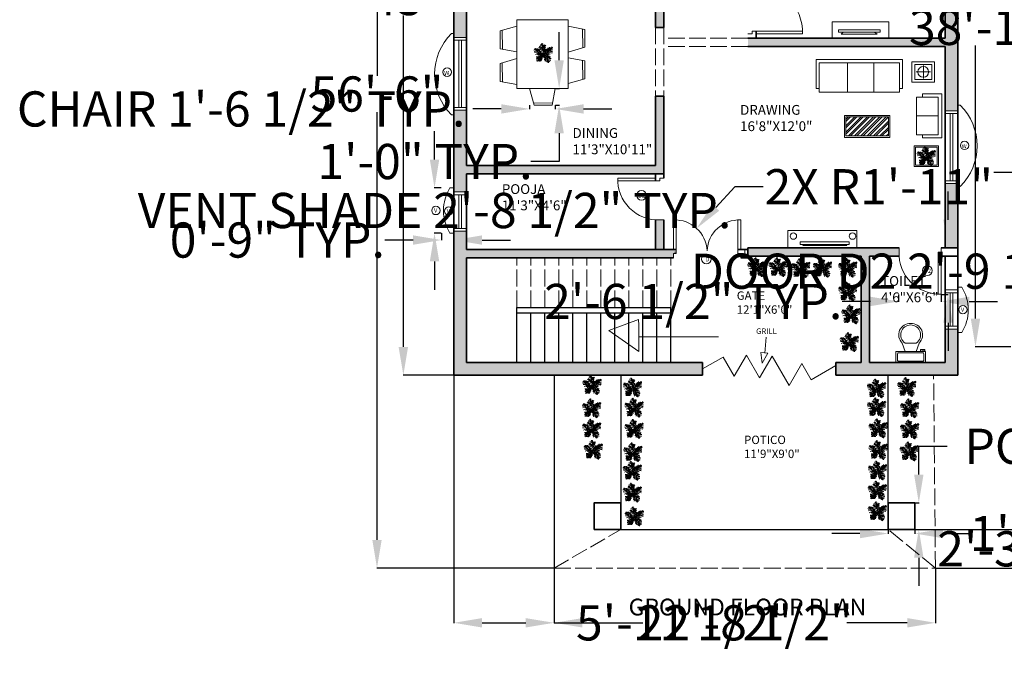
# Model space of a CAD drawing. Units: inches. Extents: x 28 to 3832, y 2 to 1709.
# Tile 1 of 7: x 2252 to 2956, y 827 to 1296. Entities that reach past the tile are written whole.
import ezdxf

# ---------------------------------------------------------------- set-up
doc = ezdxf.new("R2010")
doc.units = ezdxf.units.IN
doc.header["$MEASUREMENT"] = 0
doc.linetypes.add('ACAD_ISO02W100', pattern=[15, 12, -3])
for name, color, linetype, lineweight in [('A-ANNO-DIMS', 2, 'Continuous', 18), ('A-ANNO-SYMB', 7, 'Continuous', 13), ('A-ANNO-TEXT', 7, 'Continuous', 18), ('A-ANNO-TITL', 7, 'Continuous', 30), ('A-AREA-IDEN', 7, 'Continuous', 18), ('A-COLS', 7, 'Continuous', 35), ('A-DOOR', 3, 'Continuous', 18), ('A-FLOR-FIXT', 9, 'Continuous', 18), ('A-FLOR-PORC', 7, 'Continuous', 25), ('A-FLOR-STRS', 7, 'Continuous', 25), ('A-FLOR-STRS-OVHD', 8, 'ACAD_ISO02W100', 18), ('A-FURN', 8, 'Continuous', 18), ('A-GLAZ', 4, 'Continuous', 18), ('A-ROOF-OVHD', 8, 'ACAD_ISO02W100', 18), ('A-ROOF-SHAD', 7, 'Continuous', 13), ('A-WALL', 7, 'Continuous', 35), ('A-WALL-OVHD', 7, 'ACAD_ISO02W100', 18), ('L-PLNT', 94, 'Continuous', 13)]:
    doc.layers.add(name, color=color, linetype=linetype, lineweight=lineweight)
doc.layers.add('A-FURN-PATT', color=30, linetype='Continuous', lineweight=9, true_color=0xf26722)
doc.layers.add('A-WALL-PATT', color=30, linetype='Continuous', lineweight=9, true_color=0xf26722)
doc.styles.get("Standard").update_dxf_attribs({"font": 'arial.ttf'})
doc.dimstyles.get("Standard").update_dxf_attribs({"dimtxt": 25.18, "dimasz": 20.18, "dimexe": 0.18, "dimexo": 0.0625, "dimgap": 0.09, "dimtad": 0, "dimtih": 1, "dimtoh": 1, "dimdec": 0, "dimzin": 0, "dimdsep": 46, "dimlunit": 3, "dimtxsty": 'Standard', "dimcen": 0.09, "dimadec": 0, "dimazin": 0, "dimtfac": 1, "dimtdec": 0, "dimtofl": 0, "dimtmove": 0, "dimatfit": 3, "dimfxl": 1, "dimtolj": 1, "dimtzin": 0, "dimarcsym": 0})

# ---------------------------------------------------------------- blocks, each defined once
blk = doc.blocks.new('*D2')
at = {"layer": 'A-ANNO-DIMS', "color": 0, "lineweight": -2, "transparency": 16777216}
for p, q in [((2562.58, 1581.52), (2526.35, 1581.52)), ((2526.53, 1561.34), (2526.53, 1324.42)), ((2526.53, 1061.7), (2526.53, 1298.63)), ((2562.58, 1041.52), (2526.35, 1041.52))]:
    blk.add_line(p, q, dxfattribs=at)
at = {"layer": 'A-ANNO-DIMS', "color": 0, "transparency": 16777216}
for points in [[(2523.16, 1561.34), (2529.89, 1561.34), (2526.53, 1581.52)], [(2523.16, 1061.7), (2529.89, 1061.7), (2526.53, 1041.52)]]:
    blk.add_solid(points, dxfattribs=at)
at = {"layer": 'Defpoints', "color": 0, "transparency": 16777216}
for p in [(2562.64, 1581.52), (2526.53, 1041.52), (2562.64, 1041.52)]:
    blk.add_point(p, dxfattribs=at)
at = {"layer": 'A-ANNO-DIMS', "color": 0, "transparency": 16777216, "insert": (2526.53, 1311.52), "char_height": 25.18, "attachment_point": 5}
blk.add_mtext("\\A1;45'", dxfattribs=at)
blk = doc.blocks.new('*U6')
for p, q in [((-10.186, 53.64), (-13.084, 55.962)), ((0, 0), (-10.5, 57)), ((-9.099, 51.782), (-6.563, 55.962)), ((-47.498, 19.737), (-55.83, 18.344)), ((-40.615, 13.7), (-55.105, 10.913)), ((-31.5, 4.5), (-52.5, 25.5)), ((-33.37, 6.269), (-52.207, 5.34)), ((-48.585, 21.131), (-49.309, 29.026)), ((-28.299, 3.483), (-47.86, -5.805)), ((-43.513, 28.561), (-42.427, 15.558)), ((-38.442, 26.239), (-34.819, 7.663)), ((-21.416, 3.018), (-38.079, -8.128)), ((-35.544, 28.097), (-24.314, 3.947)), ((0, 0), (-31.5, 4.5)), ((-14.533, 2.09), (-30.834, 25.31)), ((-15.982, 2.09), (-30.11, -9.521)), ((-3.665, 19.273), (-27.574, 35.527)), ((-5.114, 28.097), (-24.676, 40.636)), ((-24.314, 23.917), (-2.941, 13.7)), ((0, 0), (-22.5, -19.5)), ((-7.288, 39.707), (-21.778, 46.673)), ((-6.563, 1.161), (-21.416, -8.128)), ((-20.691, 13.7), (-1.129, 4.876)), ((-8.737, 47.138), (-17.069, 52.711)), ((-7.65, 43.423), (-2.578, 49.46)), ((-5.839, 35.992), (4.667, 48.067)), ((-5.114, 27.632), (10.463, 46.673)), ((-2.941, 16.486), (8.652, 37.85)), ((-1.129, 6.734), (9.014, 26.704)), ((0, 0), (27, 9)), ((0, 0), (18, -22.5)), ((3.942, 1.625), (11.187, 24.381)), ((6.478, 1.625), (26.04, -8.592)), ((10.101, 3.483), (17.708, 26.239)), ((11.187, 3.483), (30.749, -5.805)), ((16.259, 5.805), (23.142, 31.348)), ((18.07, 5.805), (35.096, -3.483)), ((22.055, 7.198), (27.489, 32.277)), ((24.229, 7.663), (46.688, 1.625)), ((27, 9), (48, 36)), ((27.127, 9.056), (31.112, 35.992)), ((29.662, 12.307), (48.137, 6.269)), ((31.836, 30.883), (32.561, 16.486)), ((33.285, 16.486), (48.862, 10.913)), ((35.096, 32.741), (37.27, 22.524)), ((36.183, 19.737), (48.137, 17.88)), ((38.719, 34.134), (41.979, 28.561)), ((40.53, 25.775), (48.862, 24.846)), ((43.791, 29.954), (51.036, 30.883)), ((44.153, 36.456), (45.239, 32.741)), ((-17.431, -15.094), (-42.789, -18.809)), ((-28.299, -29.026), (-42.789, -31.348)), ((-24.314, -21.596), (-42.427, -22.06)), ((-30.834, -34.135), (-42.427, -35.528)), ((-34.457, -39.708), (-40.978, -42.494)), ((-26.849, -26.24), (-40.253, -25.775)), ((-22.5, -19.5), (-37.5, -45)), ((-32.646, -36.921), (-31.921, -44.352)), ((-15.257, -12.772), (-30.11, -12.772)), ((-29.023, -30.884), (-27.936, -43.887)), ((-25.038, -23.918), (-22.865, -45.281)), ((-20.691, -18.345), (-17.793, -44.352)), ((-6.563, -5.805), (-19.967, -9.985)), ((-17.069, -15.094), (-12.721, -40.172)), ((-13.446, -11.378), (-8.737, -32.741)), ((-9.461, -8.592), (-6.201, -23.453)), ((-4.752, -3.483), (-3.665, -14.629)), ((2.493, -3.019), (-1.491, -20.202)), ((1.769, -2.555), (24.229, -9.521)), ((5.029, -6.27), (2.131, -25.775)), ((9.014, -11.378), (3.58, -35.992)), ((14.085, -16.951), (6.478, -40.172)), ((7.565, -9.056), (32.198, -14.629)), ((18.07, -22.524), (8.289, -45.745)), ((12.274, -15.094), (36.907, -18.809)), ((20.244, -30.419), (15.897, -44.816)), ((16.259, -19.738), (36.183, -22.989)), ((18, -22.5), (27, -52.5)), ((18.433, -22.524), (40.53, -29.026)), ((19.157, -25.311), (38.719, -33.206)), ((22.78, -37.85), (19.519, -48.532)), ((21.331, -32.741), (39.081, -40.636)), ((22.78, -38.314), (34.372, -44.816)), ((24.591, -45.745), (23.142, -50.854)), ((24.591, -43.423), (30.749, -47.603)), ((26.764, -49.925), (28.213, -50.854))]:
    blk.add_line(p, q)
blk = doc.blocks.new('*U4')
for p, q in [((9.5, -6), (9.5, -2)), ((-10, -8.5), (-8, -8.5)), ((-10, -9.5), (-10, -8.5)), ((-7, -9.5), (-10, -9.5)), ((-8, -8.5), (-8, -8)), ((-7, -8), (-7, -9.5)), ((-4, -8), (-6, -14)), ((4, -14), (-4, -14)), ((4, -8), (6, -14))]:
    blk.add_line(p, q)
blk.add_lwpolyline([(10.5, -8), (10.5, 0), (-10.5, 0), (-10.5, -8)], close=True)
for points in [[(-9.5, -2), (-9.5, -6)], [(8.5, -1), (-8.5, -1)], [(-8.5, -7), (8.5, -7)]]:
    blk.add_lwpolyline(points)
for centre, radius, start, end in [((-8.625, -1.875), 0.8839, 81.8699, 188.1301), ((-8.625, -6.125), 0.8839, 171.869898, 278.1301), ((8.625, -1.875), 0.8839, 351.8699, 98.1301), ((8.625, -6.125), 0.8839, 261.8699, 8.1301), ((-0.4772, -19.9188), 8.0953, 133.01722, 273.38), ((0.0374, -19.8731), 7.127, 124.50543, 269.7), ((-0.0373, -19.8731), 7.127, 270.3, 55.4946), ((0.4773, -19.9188), 8.0953, 266.62, 46.9828)]:
    blk.add_arc(centre, radius, start, end)
blk = doc.blocks.new('DOOR-D1-36')
for p, q in [((33.01, 36), (39.01, 36)), ((36.01, 2), (0.01, 2)), ((33.01, 0), (0.01, 0)), ((36.01, 2), (36.01, 0)), ((36.01, 0), (39.01, 0))]:
    blk.add_line(p, q)
blk.add_arc((35.01, 1), 35.01, 88.36342, 181.63658)
blk = doc.blocks.new('DOOR-D2-30')
for p, q in [((0, 6), (0, 33)), ((2, 3), (2, 33)), ((2, 3), (0, 3)), ((0, 3), (0, 0)), ((30, 6), (30, 0))]:
    blk.add_line(p, q)
blk.add_arc((1, 4), 29.02, 358.02507, 91.97493)
blk = doc.blocks.new('WINDOW-48')
for p, q in [((0, 0), (0, 9)), ((2, 0), (2, 9)), ((50, 0), (50, 9)), ((52, 0), (52, 9)), ((2, 5.5), (50, 5.5)), ((2, 3.5), (50, 3.5))]:
    blk.add_line(p, q)
blk = doc.blocks.new('VENT-24')
for p, q in [((0, 0), (0, 9)), ((2, 0), (2, 9)), ((26, 0), (26, 9)), ((28, 0), (28, 9)), ((2, 5.5), (26, 5.5)), ((2, 3.5), (26, 3.5))]:
    blk.add_line(p, q)
blk = doc.blocks.new('WINDOW-SHADE')
for p, q in [((0, 1.76), (0, 0)), ((58.03, 1.76), (58.03, 0))]:
    blk.add_line(p, q)
blk.add_arc((29.02, -27.22), 41.01, 44.95711, 135.04289)
blk = doc.blocks.new('VENT-SHADE')
for p, q in [((0, 2.83), (0, 0)), ((32.5, 2.83), (32.5, 0))]:
    blk.add_line(p, q)
blk.add_arc((16.25, -23.61), 31.04, 58.4311, 121.5689)
blk = doc.blocks.new('CHAIR-DINING')
for p, q in [((0, 0), (2.18, 11.87)), ((1.91, 10.35), (15.39, 10.45)), ((2.18, 11.87), (14.98, 11.87)), ((14.98, 11.87), (18.42, 0))]:
    blk.add_line(p, q)
blk = doc.blocks.new('PORTICO-COLUMN')
blk.add_lwpolyline([(0, 0), (18.98, 0), (18.98, 19.12), (0, 19.12)], close=True)
blk = doc.blocks.new('OPENING-TAG-W')
blk.add_circle((3, 3), 3)
at = {"insert": (0.88, 3.88), "char_height": 3, "attachment_point": 1}
blk.add_mtext_dynamic_manual_height_columns('W', width=16.2124, gutter_width=1, heights=[0], dxfattribs=at)
blk = doc.blocks.new('OPENING-TAG-V')
blk.add_circle((3, 3), 3)
at = {"insert": (1.61, 4.52), "char_height": 3, "attachment_point": 1}
blk.add_mtext_dynamic_manual_height_columns('V', width=16.2124, gutter_width=1, heights=[0], dxfattribs=at)
blk = doc.blocks.new('OPENING-TAG-D2')
blk.add_circle((3.43, 3.43), 3.43)
at = {"insert": (0.96, 4.81), "char_height": 3, "attachment_point": 1}
blk.add_mtext_dynamic_manual_height_columns('D2', width=16.2124, gutter_width=1, heights=[0], dxfattribs=at)
blk = doc.blocks.new('*D27')
at = {"layer": 'A-ANNO-DIMS', "color": 0, "lineweight": -2, "transparency": 16777216}
for p, q in [((2596.46, 1231.9), (2576.28, 1231.9)), ((2616.64, 1234.6), (2616.64, 1231.72)), ((2635.06, 1234.6), (2635.06, 1231.72)), ((2655.24, 1231.9), (2675.42, 1231.9))]:
    blk.add_line(p, q, dxfattribs=at)
at = {"layer": 'A-ANNO-DIMS', "color": 0, "transparency": 16777216}
for points in [[(2596.46, 1235.27), (2596.46, 1228.54), (2616.64, 1231.9)], [(2655.24, 1235.27), (2655.24, 1228.54), (2635.06, 1231.9)]]:
    blk.add_solid(points, dxfattribs=at)
at = {"layer": 'Defpoints', "color": 0, "transparency": 16777216}
for p in [(2616.64, 1234.67), (2616.64, 1231.9), (2635.06, 1234.67)]:
    blk.add_point(p, dxfattribs=at)
at = {"layer": 'A-ANNO-DIMS', "color": 0, "transparency": 16777216, "insert": (2410.65, 1231.9), "char_height": 25.18, "attachment_point": 5}
blk.add_mtext('\\A1;CHAIR 1\'-6 1/2" TYP.', dxfattribs=at)
blk = doc.blocks.new('*D28')
at = {"layer": 'A-ANNO-DIMS', "color": 0, "lineweight": -2, "transparency": 16777216}
for p, q in [((2637.82, 1266.72), (2637.82, 1286.9)), ((2635.12, 1246.54), (2638, 1246.54)), ((2635.12, 1234.67), (2638, 1234.67)), ((2637.82, 1214.49), (2637.82, 1194.31)), ((2637.82, 1194.31), (2617.64, 1194.31))]:
    blk.add_line(p, q, dxfattribs=at)
at = {"layer": 'A-ANNO-DIMS', "color": 0, "transparency": 16777216}
for points in [[(2634.46, 1266.72), (2641.18, 1266.72), (2637.82, 1246.54)], [(2634.46, 1214.49), (2641.18, 1214.49), (2637.82, 1234.67)]]:
    blk.add_solid(points, dxfattribs=at)
at = {"layer": 'Defpoints', "color": 0, "transparency": 16777216}
for p in [(2635.06, 1246.54), (2635.06, 1234.67), (2637.82, 1234.67)]:
    blk.add_point(p, dxfattribs=at)
at = {"layer": 'A-ANNO-DIMS', "color": 0, "transparency": 16777216, "insert": (2541.99, 1194.31), "char_height": 25.18, "attachment_point": 5}
blk.add_mtext('\\A1;1\'-0" TYP.', dxfattribs=at)
blk = doc.blocks.new('*D29')
at = {"layer": 'A-ANNO-DIMS', "color": 0, "lineweight": -2, "transparency": 16777216}
for p, q in [((2968.49, 1186.57), (2948.31, 1186.57)), ((2988.67, 1181.34), (2988.67, 1186.75)), ((3023.98, 1181.34), (3023.98, 1186.75)), ((3044.16, 1186.57), (3064.34, 1186.57))]:
    blk.add_line(p, q, dxfattribs=at)
at = {"layer": 'A-ANNO-DIMS', "color": 0, "transparency": 16777216}
for points in [[(2968.49, 1189.93), (2968.49, 1183.21), (2988.67, 1186.57)], [(3044.16, 1189.93), (3044.16, 1183.21), (3023.98, 1186.57)]]:
    blk.add_solid(points, dxfattribs=at)
at = {"layer": 'Defpoints', "color": 0, "transparency": 16777216}
for p in [(3023.98, 1186.57), (2988.67, 1181.27), (3023.98, 1181.27)]:
    blk.add_point(p, dxfattribs=at)
at = {"layer": 'A-ANNO-DIMS', "color": 0, "transparency": 16777216, "insert": (3305.33, 1186.57), "char_height": 25.18, "attachment_point": 5}
blk.add_mtext('\\A1;SIDE CANOPY 2\'-11 1/2" TYP.', dxfattribs=at)
blk = doc.blocks.new('*D33')
at = {"layer": 'A-ANNO-DIMS', "color": 0, "lineweight": -2, "transparency": 16777216}
for p, q in [((2915.63, 1152.7), (2915.63, 1172.88)), ((2910.7, 1132.52), (2915.81, 1132.52)), ((2910.7, 1099.25), (2915.81, 1099.25)), ((2915.63, 1079.07), (2915.63, 1058.89))]:
    blk.add_line(p, q, dxfattribs=at)
at = {"layer": 'A-ANNO-DIMS', "color": 0, "transparency": 16777216}
for points in [[(2912.27, 1152.7), (2918.99, 1152.7), (2915.63, 1132.52)], [(2912.27, 1079.07), (2918.99, 1079.07), (2915.63, 1099.25)]]:
    blk.add_solid(points, dxfattribs=at)
at = {"layer": 'Defpoints', "color": 0, "transparency": 16777216}
for p in [(2910.64, 1132.52), (2910.64, 1099.25), (2915.63, 1099.25)]:
    blk.add_point(p, dxfattribs=at)
at = {"layer": 'A-ANNO-DIMS', "color": 0, "transparency": 16777216, "insert": (2915.63, 1115.88), "char_height": 25.18, "attachment_point": 5}
blk.add_mtext('\\A1;DOOR D2 2\'-9 1/2" TYP.', dxfattribs=at)
blk = doc.blocks.new('*D34')
at = {"layer": 'A-ANNO-DIMS', "color": 0, "lineweight": -2, "transparency": 16777216}
for p, q in [((2880.36, 1099.18), (2880.36, 1094.07)), ((2910.64, 1099.18), (2910.64, 1094.07)), ((2860.18, 1094.25), (2840, 1094.25)), ((2930.82, 1094.25), (2951, 1094.25))]:
    blk.add_line(p, q, dxfattribs=at)
at = {"layer": 'A-ANNO-DIMS', "color": 0, "transparency": 16777216}
for points in [[(2860.18, 1097.62), (2860.18, 1090.89), (2880.36, 1094.25)], [(2930.82, 1097.62), (2930.82, 1090.89), (2910.64, 1094.25)]]:
    blk.add_solid(points, dxfattribs=at)
at = {"layer": 'Defpoints', "color": 0, "transparency": 16777216}
for p in [(2880.36, 1099.25), (2910.64, 1099.25), (2880.36, 1094.25)]:
    blk.add_point(p, dxfattribs=at)
at = {"layer": 'A-ANNO-DIMS', "color": 0, "transparency": 16777216, "insert": (2733.62, 1094.25), "char_height": 25.18, "attachment_point": 5}
blk.add_mtext('\\A1;2\'-6 1/2" TYP.', dxfattribs=at)
blk = doc.blocks.new('*D37')
at = {"layer": 'A-ANNO-DIMS', "color": 0, "lineweight": -2, "transparency": 16777216}
for p, q in [((2548.81, 1195.71), (2548.81, 1215.89)), ((2553.62, 1175.53), (2548.63, 1175.53)), ((2553.62, 1143.04), (2548.63, 1143.04)), ((2548.81, 1122.86), (2548.81, 1102.68))]:
    blk.add_line(p, q, dxfattribs=at)
at = {"layer": 'A-ANNO-DIMS', "color": 0, "transparency": 16777216}
for points in [[(2545.44, 1195.71), (2552.17, 1195.71), (2548.81, 1175.53)], [(2545.44, 1122.86), (2552.17, 1122.86), (2548.81, 1143.04)]]:
    blk.add_solid(points, dxfattribs=at)
at = {"layer": 'Defpoints', "color": 0, "transparency": 16777216}
for p in [(2548.81, 1175.53), (2553.68, 1175.53), (2553.68, 1143.04)]:
    blk.add_point(p, dxfattribs=at)
at = {"layer": 'A-ANNO-DIMS', "color": 0, "transparency": 16777216, "insert": (2548.81, 1159.29), "char_height": 25.18, "attachment_point": 5}
blk.add_mtext('\\A1;VENT SHADE 2\'-8 1/2" TYP.', dxfattribs=at)
blk = doc.blocks.new('*D38')
at = {"layer": 'A-ANNO-DIMS', "color": 0, "lineweight": -2, "transparency": 16777216}
for p, q in [((2553.68, 1142.97), (2553.68, 1137.98)), ((2562.64, 1142.97), (2562.64, 1137.98)), ((2533.5, 1138.16), (2513.32, 1138.16)), ((2582.82, 1138.16), (2603, 1138.16))]:
    blk.add_line(p, q, dxfattribs=at)
at = {"layer": 'A-ANNO-DIMS', "color": 0, "transparency": 16777216}
for points in [[(2533.5, 1141.52), (2533.5, 1134.8), (2553.68, 1138.16)], [(2582.82, 1141.52), (2582.82, 1134.8), (2562.64, 1138.16)]]:
    blk.add_solid(points, dxfattribs=at)
at = {"layer": 'Defpoints', "color": 0, "transparency": 16777216}
for p in [(2553.68, 1143.04), (2562.64, 1143.04), (2553.68, 1138.16)]:
    blk.add_point(p, dxfattribs=at)
at = {"layer": 'A-ANNO-DIMS', "color": 0, "transparency": 16777216, "insert": (2436.49, 1138.16), "char_height": 25.18, "attachment_point": 5}
blk.add_mtext('\\A1;0\'-9" TYP.', dxfattribs=at)
blk = doc.blocks.new('*D43')
at = {"layer": 'A-ANNO-DIMS', "color": 0, "lineweight": -2, "transparency": 16777216}
for p, q in [((2894.75, 970.5), (2894.75, 990.68)), ((2894.75, 990.68), (2914.93, 990.68)), ((2891.95, 950.32), (2894.93, 950.32)), ((2891.95, 931.2), (2894.93, 931.2)), ((2894.75, 911.02), (2894.75, 890.84))]:
    blk.add_line(p, q, dxfattribs=at)
at = {"layer": 'A-ANNO-DIMS', "color": 0, "transparency": 16777216}
for points in [[(2891.39, 970.5), (2898.12, 970.5), (2894.75, 950.32)], [(2891.39, 911.02), (2898.12, 911.02), (2894.75, 931.2)]]:
    blk.add_solid(points, dxfattribs=at)
at = {"layer": 'Defpoints', "color": 0, "transparency": 16777216}
for p in [(2891.88, 950.32), (2894.75, 950.32), (2891.88, 931.2)]:
    blk.add_point(p, dxfattribs=at)
at = {"layer": 'A-ANNO-DIMS', "color": 0, "transparency": 16777216, "insert": (3157.26, 990.68), "char_height": 25.18, "attachment_point": 5}
blk.add_mtext('\\A1;PORTICO COLUMN 1\'-7" TYP.', dxfattribs=at)
blk = doc.blocks.new('*D44')
at = {"layer": 'A-ANNO-DIMS', "color": 0, "lineweight": -2, "transparency": 16777216}
for p, q in [((2872.9, 931.14), (2872.9, 928.15)), ((2891.88, 931.14), (2891.88, 928.15)), ((2852.72, 928.33), (2832.54, 928.33)), ((2912.06, 928.33), (2932.24, 928.33))]:
    blk.add_line(p, q, dxfattribs=at)
at = {"layer": 'A-ANNO-DIMS', "color": 0, "transparency": 16777216}
for points in [[(2852.72, 931.69), (2852.72, 924.97), (2872.9, 928.33)], [(2912.06, 931.69), (2912.06, 924.97), (2891.88, 928.33)]]:
    blk.add_solid(points, dxfattribs=at)
at = {"layer": 'Defpoints', "color": 0, "transparency": 16777216}
for p in [(2872.9, 931.2), (2891.88, 931.2), (2891.88, 928.33)]:
    blk.add_point(p, dxfattribs=at)
at = {"layer": 'A-ANNO-DIMS', "color": 0, "transparency": 16777216, "insert": (3007.89, 928.33), "char_height": 25.18, "attachment_point": 5}
blk.add_mtext('\\A1;1\'-7" TYP.', dxfattribs=at)
blk = doc.blocks.new('*D47')
at = {"layer": 'A-ANNO-DIMS', "color": 0, "lineweight": -2, "transparency": 16777216}
for p, q in [((2562.58, 1581.52), (2507.53, 1581.52)), ((2507.71, 1561.34), (2507.71, 1255.51)), ((2507.71, 923.79), (2507.71, 1229.62)), ((2634.1, 903.61), (2507.53, 903.61))]:
    blk.add_line(p, q, dxfattribs=at)
at = {"layer": 'A-ANNO-DIMS', "color": 0, "transparency": 16777216}
for points in [[(2504.35, 1561.34), (2511.07, 1561.34), (2507.71, 1581.52)], [(2504.35, 923.79), (2511.07, 923.79), (2507.71, 903.61)]]:
    blk.add_solid(points, dxfattribs=at)
at = {"layer": 'Defpoints', "color": 0, "transparency": 16777216}
for p in [(2507.71, 1581.52), (2562.64, 1581.52), (2634.16, 903.61)]:
    blk.add_point(p, dxfattribs=at)
at = {"layer": 'A-ANNO-DIMS', "color": 0, "transparency": 16777216, "insert": (2507.71, 1242.57), "char_height": 25.18, "attachment_point": 5}
blk.add_mtext('\\A1;56\'-6"', dxfattribs=at)
blk = doc.blocks.new('*D48')
at = {"layer": 'A-ANNO-DIMS', "color": 0, "lineweight": -2, "transparency": 16777216}
for p, q in [((2634.16, 903.55), (2634.16, 864.33)), ((2906.67, 903.55), (2906.67, 864.33)), ((2654.34, 864.51), (2697.53, 864.51)), ((2886.49, 864.51), (2843.31, 864.51))]:
    blk.add_line(p, q, dxfattribs=at)
at = {"layer": 'A-ANNO-DIMS', "color": 0, "transparency": 16777216}
for points in [[(2654.34, 867.87), (2654.34, 861.15), (2634.16, 864.51)], [(2886.49, 867.87), (2886.49, 861.15), (2906.67, 864.51)]]:
    blk.add_solid(points, dxfattribs=at)
at = {"layer": 'Defpoints', "color": 0, "transparency": 16777216}
for p in [(2634.16, 903.61), (2906.67, 903.61), (2906.67, 864.51)]:
    blk.add_point(p, dxfattribs=at)
at = {"layer": 'A-ANNO-DIMS', "color": 0, "transparency": 16777216, "insert": (2770.42, 864.51), "char_height": 25.18, "attachment_point": 5}
blk.add_mtext('\\A1;22\'-8 1/2"', dxfattribs=at)
blk = doc.blocks.new('*D49')
at = {"layer": 'A-ANNO-DIMS', "color": 0, "lineweight": -2, "transparency": 16777216}
for p, q in [((2562.64, 1041.46), (2562.64, 864.33)), ((2634.16, 1041.46), (2634.16, 864.33)), ((2582.82, 864.51), (2613.98, 864.51)), ((2634.16, 864.51), (2654.34, 864.51))]:
    blk.add_line(p, q, dxfattribs=at)
at = {"layer": 'A-ANNO-DIMS', "color": 0, "transparency": 16777216}
for points in [[(2582.82, 867.87), (2582.82, 861.15), (2562.64, 864.51)], [(2613.98, 867.87), (2613.98, 861.15), (2634.16, 864.51)]]:
    blk.add_solid(points, dxfattribs=at)
at = {"layer": 'Defpoints', "color": 0, "transparency": 16777216}
for p in [(2562.64, 1041.52), (2634.16, 1041.52), (2634.16, 864.51)]:
    blk.add_point(p, dxfattribs=at)
at = {"layer": 'A-ANNO-DIMS', "color": 0, "transparency": 16777216, "insert": (2727.01, 864.51), "char_height": 25.18, "attachment_point": 5}
blk.add_mtext('\\A1;5\'-11 1/2"', dxfattribs=at)
blk = doc.blocks.new('*D52')
at = {"layer": 'A-ANNO-DIMS', "color": 0, "lineweight": -2, "transparency": 16777216}
for p, q in [((2975.53, 951.38), (2975.53, 971.56)), ((2891.95, 931.2), (2975.71, 931.2)), ((2906.74, 903.61), (2975.71, 903.61)), ((2975.53, 883.43), (2975.53, 863.25))]:
    blk.add_line(p, q, dxfattribs=at)
at = {"layer": 'A-ANNO-DIMS', "color": 0, "transparency": 16777216}
for points in [[(2972.16, 951.38), (2978.89, 951.38), (2975.53, 931.2)], [(2972.16, 883.43), (2978.89, 883.43), (2975.53, 903.61)]]:
    blk.add_solid(points, dxfattribs=at)
at = {"layer": 'Defpoints', "color": 0, "transparency": 16777216}
for p in [(2891.88, 931.2), (2975.53, 931.2), (2906.67, 903.61)]:
    blk.add_point(p, dxfattribs=at)
at = {"layer": 'A-ANNO-DIMS', "color": 0, "transparency": 16777216, "insert": (2975.53, 917.41), "char_height": 25.18, "attachment_point": 5}
blk.add_mtext('\\A1;2\'-3 1/2"', dxfattribs=at)
blk = doc.blocks.new('*D54')
at = {"layer": 'A-ANNO-DIMS', "color": 0, "lineweight": -2, "transparency": 16777216}
for p, q in [((3022.59, 1518.63), (2935.04, 1518.63)), ((2935.22, 1498.45), (2935.22, 1303.17)), ((2935.22, 1081.98), (2935.22, 1277.26)), ((2960.61, 1061.8), (2935.04, 1061.8))]:
    blk.add_line(p, q, dxfattribs=at)
at = {"layer": 'A-ANNO-DIMS', "color": 0, "transparency": 16777216}
for points in [[(2931.86, 1498.45), (2938.58, 1498.45), (2935.22, 1518.63)], [(2931.86, 1081.98), (2938.58, 1081.98), (2935.22, 1061.8)]]:
    blk.add_solid(points, dxfattribs=at)
at = {"layer": 'Defpoints', "color": 0, "transparency": 16777216}
for p in [(2935.22, 1518.63), (3022.65, 1518.63), (2960.67, 1061.8)]:
    blk.add_point(p, dxfattribs=at)
at = {"layer": 'A-ANNO-DIMS', "color": 0, "transparency": 16777216, "insert": (2935.22, 1290.21), "char_height": 25.18, "attachment_point": 5}
blk.add_mtext('\\A1;38\'-1"', dxfattribs=at)
blk = doc.blocks.new('*D71')
at = {"layer": 'A-ANNO-DIMS', "color": 0, "lineweight": -2, "transparency": 16777216}
for p, q in [((2763.33, 1176.25), (2749.7, 1161.37)), ((2783.51, 1176.25), (2763.33, 1176.25)), ((2720.41, 1129.52), (2720.59, 1129.52)), ((2720.5, 1129.43), (2720.5, 1129.61))]:
    blk.add_line(p, q, dxfattribs=at)
at = {"layer": 'A-ANNO-DIMS', "color": 0, "transparency": 16777216}
blk.add_solid([(2747.22, 1163.64), (2752.18, 1159.1), (2736.06, 1146.49)], dxfattribs=at)
at = {"layer": 'Defpoints', "color": 0, "transparency": 16777216}
for p in [(2736.06, 1146.49), (2720.5, 1129.52)]:
    blk.add_point(p, dxfattribs=at)
at = {"layer": 'A-ANNO-DIMS', "color": 0, "transparency": 16777216, "insert": (2866.17, 1176.25), "char_height": 25.18, "attachment_point": 5}
blk.add_mtext('\\A1;2X R1\'-11"', dxfattribs=at)

msp = doc.modelspace()

# ---------------------------------------------------------------- hatches: boundary and pattern name
at = {"layer": 'A-FURN-PATT'}
h = msp.add_hatch(dxfattribs=at)
h.set_pattern_fill('ANSI32', color=256, scale=8.5)
h.paths.add_polyline_path([(2873.03, 1226.16), (2842.71, 1226.16), (2842.71, 1212.59), (2873.03, 1212.59)])
at = {"layer": 'A-WALL-PATT'}
h = msp.add_hatch(color=256, dxfattribs=at)
h.dxf.hatch_style = 1
h.paths.add_polyline_path([(2571.64, 1572.52), (2613.14, 1572.52), (2613.14, 1581.52), (2562.64, 1581.52), (2562.64, 1527.52), (2571.64, 1527.52)])
h.paths.add_polyline_path([(2728.64, 1581.52), (2665.14, 1581.52), (2665.14, 1572.52), (2670.22, 1572.52), (2706.64, 1572.52), (2706.64, 1469.52), (2707.64, 1469.52, -0.014283), (2709.64, 1469.52), (2712.64, 1469.52), (2712.64, 1471.52), (2712.64, 1477.52), (2712.64, 1572.52), (2728.64, 1572.52)])
h.paths.add_polyline_path([(2820.14, 1581.52), (2756.64, 1581.52), (2756.64, 1572.52), (2772.64, 1572.52), (2772.64, 1477.52), (2745.64, 1477.52), (2745.64, 1476.52, -0.017236), (2745.64, 1474.52), (2745.64, 1471.52), (2772.64, 1471.52), (2772.64, 1469.52), (2775.64, 1469.52, -0.006113), (2776.49, 1469.52), (2778.64, 1469.52), (2778.64, 1572.52), (2820.14, 1572.52)])
h.paths.add_polyline_path([(2922.64, 1581.52), (2872.14, 1581.52), (2872.14, 1572.52), (2913.64, 1572.52), (2913.64, 1527.52), (2922.64, 1527.52)])
h.paths.add_polyline_path([(2922.64, 1475.52), (2913.64, 1475.52), (2913.64, 1430.52), (2778.64, 1430.52), (2772.64, 1430.52), (2772.64, 1321.52), (2775.64, 1321.52, -0.014283), (2777.64, 1321.52), (2778.64, 1321.52), (2778.64, 1424.52), (2913.64, 1424.52), (2913.64, 1379.52), (2922.64, 1379.52)])
h.paths.add_polyline_path([(2571.64, 1475.52), (2562.64, 1475.52), (2562.64, 1402.52), (2571.64, 1402.52), (2571.64, 1424.52), (2706.64, 1424.52), (2706.64, 1328.52), (2706.64, 1322.52), (2706.64, 1290.16), (2712.64, 1290.16), (2712.64, 1430.52), (2706.64, 1430.52), (2571.64, 1430.52)])
h.paths.add_polyline_path([(2571.64, 1322.52), (2667.64, 1322.52), (2667.64, 1325.52, -0.014283), (2667.64, 1327.52), (2667.64, 1328.52), (2571.64, 1328.52), (2571.64, 1350.52), (2562.64, 1350.52), (2562.64, 1283.02), (2571.64, 1283.02)])
h.paths.add_polyline_path([(2712.64, 1241.01), (2706.64, 1241.01), (2706.64, 1191.52), (2571.64, 1191.52), (2571.64, 1231.02), (2562.64, 1231.02), (2562.64, 1172.52), (2571.64, 1172.52), (2571.64, 1185.52), (2706.64, 1185.52), (2712.64, 1185.52)])
h.paths.add_polyline_path([(2571.64, 1125.52), (2712.64, 1125.52), (2719.5, 1125.52), (2719.5, 1128.52), (2721.5, 1128.52), (2721.5, 1131.52), (2571.64, 1131.52), (2571.64, 1144.52), (2562.64, 1144.52), (2562.64, 1041.52), (2740.31, 1041.52), (2740.31, 1050.52), (2571.64, 1050.52)])
h.paths.add_polyline_path([(2712.64, 1152.52), (2709.64, 1152.52, -0.017236), (2707.64, 1152.52), (2706.64, 1152.52), (2706.64, 1131.52), (2712.64, 1131.52)])
h.paths.add_polyline_path([(2922.64, 1178.52), (2913.64, 1178.52), (2913.64, 1132.52), (2922.64, 1132.52)], flags=17)
h.paths.add_polyline_path([(2922.64, 1327.52), (2913.64, 1327.52), (2913.64, 1282.52), (2772.64, 1282.52), (2772.64, 1276.52), (2778.64, 1276.52), (2913.64, 1276.52), (2913.64, 1230.52), (2922.64, 1230.52)])
edge = h.paths.add_edge_path()
edge.add_line((2880.64, 1132.52), (2772.64, 1132.52))
edge.add_line((2772.64, 1132.52), (2772.64, 1126.52))
edge.add_line((2772.64, 1126.52), (2853.64, 1126.52))
edge.add_line((2853.64, 1126.52), (2853.64, 1050.52))
edge.add_line((2853.64, 1050.52), (2835.37, 1050.52))
edge.add_line((2835.37, 1050.52), (2835.37, 1041.52))
edge.add_line((2835.37, 1041.52), (2922.64, 1041.52))
edge.add_line((2922.64, 1041.52), (2922.64, 1074.52))
edge.add_line((2922.64, 1074.52), (2913.64, 1074.52))
edge.add_line((2913.64, 1074.52), (2913.64, 1050.52))
edge.add_line((2913.64, 1050.52), (2859.64, 1050.52))
edge.add_line((2859.64, 1050.52), (2859.64, 1126.52))
edge.add_line((2859.64, 1126.52), (2880.64, 1126.52))
edge.add_line((2880.64, 1126.52), (2880.64, 1127.52))
edge.add_arc((2909.64, 1128.52), 29.02, 178.02507, 181.97493, ccw=False)
edge.add_line((2880.64, 1129.52), (2880.64, 1132.52))

# ---------------------------------------------------------------- linework, layer by layer
at = {"layer": 'A-ANNO-SYMB'}
for p, q in [((2673.4, 1073.44), (2694.58, 1081.31)), ((2694.58, 1081.31), (2694.74, 1077.41)), ((2694.74, 1068.97), (2694.74, 1077.41)), ((2694.74, 1077.41), (2694.74, 1058.37)), ((2694.74, 1058.37), (2673.4, 1073.44)), ((2751.73, 1068.97), (2694.74, 1068.97))]:
    msp.add_line(p, q, dxfattribs=at)
msp.add_circle((2743.02, 1124.54), 3.43, dxfattribs=at)
at = {"layer": 'A-ANNO-TEXT'}
for p, q in [((2785.78, 1068.77), (2784.77, 1057.39)), ((2781.85, 1057.7), (2786.86, 1057.17)), ((2782.94, 1050.04), (2781.85, 1057.7)), ((2786.86, 1057.17), (2782.94, 1050.04))]:
    msp.add_line(p, q, dxfattribs=at)
at = {"layer": 'A-DOOR'}
for p, q in [((2719.5, 1131.52), (2719.5, 1152.52)), ((2721.5, 1128.52), (2721.5, 1152.52)), ((2765.5, 1128.52), (2765.5, 1152.52)), ((2767.5, 1131.52), (2767.5, 1152.52)), ((2719.5, 1125.52), (2719.5, 1128.52)), ((2721.5, 1128.52), (2719.5, 1128.52)), ((2743.44, 1131.52), (2743.57, 1131.52)), ((2743.5, 1130.52), (2743.5, 1131.52)), ((2765.5, 1128.52), (2767.5, 1128.52)), ((2767.5, 1125.52), (2767.5, 1128.52)), ((2770.5, 1125.52), (2770.5, 1131.52)), ((2762.88, 1040.83), (2771.58, 1055.9)), ((2771.58, 1055.9), (2781.01, 1039.57)), ((2781.01, 1039.57), (2790, 1055.15)), ((2790, 1055.15), (2802.18, 1034.07)), ((2740.31, 1046.02), (2754.99, 1054.5)), ((2754.99, 1054.5), (2762.88, 1040.83)), ((2802.18, 1034.07), (2811.27, 1049.81)), ((2811.27, 1049.81), (2817.91, 1038.31)), ((2817.91, 1038.31), (2835.37, 1048.4))]:
    msp.add_line(p, q, dxfattribs=at)
for centre, start, end in [((2720.5, 1129.52), 2.48955, 92.48955), ((2766.5, 1129.52), 87.51045, 177.51045)]:
    msp.add_arc(centre, 23.02, start, end, dxfattribs=at)
at = {"layer": 'A-FLOR-PORC'}
for p, q in [((2681.84, 1041.52), (2681.84, 931.2)), ((2872.9, 931.2), (2872.9, 1041.52)), ((2681.84, 931.2), (2872.9, 931.2))]:
    msp.add_line(p, q, dxfattribs=at)
at = {"layer": 'A-FLOR-STRS'}
for p, q in [((2607.64, 1050.52), (2607.64, 1090.02)), ((2607.64, 1090.02), (2717.64, 1090.02)), ((2607.64, 1086.02), (2717.64, 1086.02)), ((2617.64, 1050.52), (2617.64, 1086.02)), ((2627.64, 1050.52), (2627.64, 1086.02)), ((2637.64, 1050.52), (2637.64, 1086.02)), ((2647.64, 1050.52), (2647.64, 1086.02)), ((2657.64, 1050.52), (2657.64, 1086.02)), ((2667.64, 1050.52), (2667.64, 1086.02)), ((2677.64, 1050.52), (2677.64, 1086.02)), ((2687.64, 1050.52), (2687.64, 1086.02)), ((2697.64, 1050.52), (2697.64, 1086.02)), ((2697.64, 1050.52), (2697.64, 1086.02)), ((2707.64, 1050.52), (2707.64, 1086.02)), ((2717.64, 1050.52), (2717.64, 1090.02))]:
    msp.add_line(p, q, dxfattribs=at)
at = {"layer": 'A-FLOR-STRS-OVHD'}
for p, q in [((2607.64, 1090.02), (2607.64, 1125.52)), ((2617.64, 1090.02), (2617.64, 1125.52)), ((2627.64, 1090.02), (2627.64, 1125.52)), ((2637.64, 1090.02), (2637.64, 1125.52)), ((2647.64, 1090.02), (2647.64, 1125.52)), ((2657.64, 1090.02), (2657.64, 1125.52)), ((2667.64, 1090.02), (2667.64, 1125.52)), ((2677.64, 1090.02), (2677.64, 1125.52)), ((2687.64, 1090.02), (2687.64, 1125.52)), ((2697.64, 1090.02), (2697.64, 1125.52)), ((2707.64, 1090.02), (2707.64, 1125.52)), ((2717.64, 1090.02), (2717.64, 1125.52))]:
    msp.add_line(p, q, dxfattribs=at)
at = {"layer": 'A-FURN'}
for p, q in [((2843.8, 1264.82), (2843.8, 1243.85)), ((2862.52, 1264.82), (2862.52, 1243.85)), ((2898.07, 1262.9), (2898.07, 1253.75)), ((2892.93, 1258.36), (2903.22, 1258.36)), ((2908.49, 1226.86), (2893.16, 1226.86)), ((2812.76, 1134.98), (2811.95, 1134.36)), ((2811.95, 1134.36), (2843.37, 1134.36)), ((2843.37, 1134.36), (2842.19, 1134.98))]:
    msp.add_line(p, q, dxfattribs=at)
for points in [[(2607.61, 1295.72), (2644.22, 1295.72), (2644.22, 1246.54), (2607.61, 1246.54)], [(2832.85, 1282.52), (2873.38, 1282.52), (2873.38, 1294.17), (2832.85, 1294.17)], [(2837.27, 1288.49), (2867.11, 1288.49), (2867.11, 1286.81), (2837.27, 1286.81)], [(2823.53, 1264.82), (2880.91, 1264.82), (2880.91, 1243.85), (2823.53, 1243.85)], [(2889.83, 1265.68), (2906.06, 1265.68), (2906.06, 1251.05), (2889.83, 1251.05)], [(2891.83, 1263.68), (2904.06, 1263.68), (2904.06, 1253.05), (2891.83, 1253.05)], [(2893.16, 1240.42), (2908.49, 1240.42), (2908.49, 1213.31), (2893.16, 1213.31)], [(2841.71, 1227.16), (2874.03, 1227.16), (2874.03, 1211.59), (2841.71, 1211.59)], [(2842.71, 1226.16), (2873.03, 1226.16), (2873.03, 1212.59), (2842.71, 1212.59)], [(2801.26, 1132.52), (2850.39, 1132.52), (2850.39, 1144.9), (2801.26, 1144.9)], [(2809.95, 1136.88), (2845, 1136.88), (2845, 1134.98), (2809.95, 1134.98)]]:
    msp.add_lwpolyline(points, close=True, dxfattribs=at)
for points in [[(2840.79, 1286.81), (2839.18, 1285.34), (2864.91, 1285.34), (2863.11, 1286.81)], [(2823.53, 1267.17), (2821.35, 1267.17), (2821.35, 1246.42), (2823.53, 1246.42), (2823.53, 1264.82)], [(2880.88, 1267.17), (2823.53, 1267.17)], [(2880.88, 1264.82), (2880.88, 1246.42), (2883.07, 1246.42), (2883.07, 1267.17), (2880.88, 1267.17)], [(2823.53, 1264.82), (2880.88, 1264.82)], [(2908.49, 1240.42), (2897.38, 1240.42), (2897.38, 1242.59), (2911.23, 1242.59), (2911.23, 1240.42)], [(2908.49, 1213.32), (2908.49, 1240.42)], [(2911.23, 1240.42), (2911.23, 1213.32)], [(2911.23, 1213.32), (2911.23, 1211.15), (2897.38, 1211.15), (2897.38, 1213.32), (2908.49, 1213.32)]]:
    msp.add_lwpolyline(points, dxfattribs=at)
for centre, radius in [((2897.94, 1258.36), 3.83), ((2805.15, 1141), 2.3), ((2847.38, 1141), 2.3)]:
    msp.add_circle(centre, radius, dxfattribs=at)
at = {"layer": 'A-ROOF-OVHD'}
for p, q in [((2634.16, 1041.52), (2634.16, 903.61)), ((2906.67, 903.61), (2905.32, 1041.52)), ((2634.16, 903.61), (2681.84, 931.2)), ((2906.67, 903.61), (2872.9, 931.2)), ((2634.16, 903.61), (2906.67, 903.61))]:
    msp.add_line(p, q, dxfattribs=at)
at = {"layer": 'A-WALL'}
for p, q in [((2562.64, 1041.52), (2562.64, 1581.52)), ((2922.64, 1581.52), (2922.64, 1041.52)), ((2712.64, 1290.16), (2712.64, 1433.52)), ((2913.64, 1424.52), (2913.64, 1282.52)), ((2571.64, 1191.52), (2571.64, 1322.52)), ((2706.64, 1290.16), (2706.64, 1322.52)), ((2706.64, 1290.16), (2712.64, 1290.16)), ((2778.64, 1287.52), (2778.64, 1282.52)), ((2772.64, 1282.52), (2913.64, 1282.52)), ((2913.64, 1282.52), (2772.64, 1282.52)), ((2772.64, 1276.52), (2913.64, 1276.52)), ((2913.64, 1276.52), (2913.64, 1132.52)), ((2706.64, 1191.52), (2706.64, 1241.01)), ((2706.64, 1241.01), (2712.64, 1241.01)), ((2712.64, 1182.52), (2712.64, 1241.01)), ((2571.64, 1191.52), (2706.64, 1191.52)), ((2571.64, 1185.52), (2706.64, 1185.52)), ((2571.64, 1131.52), (2571.64, 1185.52)), ((2706.64, 1185.52), (2712.64, 1185.52)), ((2706.64, 1180.52), (2706.64, 1185.52)), ((2706.64, 1131.52), (2706.64, 1152.57)), ((2712.64, 1131.52), (2712.64, 1152.52)), ((2772.64, 1132.52), (2772.64, 1126.52)), ((2778.64, 1132.52), (2772.64, 1132.52)), ((2778.64, 1132.52), (2880.64, 1132.52)), ((2910.64, 1132.52), (2913.64, 1132.52)), ((2913.64, 1132.52), (2922.64, 1132.52)), ((2571.64, 1131.52), (2721.5, 1131.52)), ((2571.64, 1050.52), (2571.64, 1125.52)), ((2571.64, 1125.52), (2712.64, 1125.52)), ((2712.64, 1125.52), (2719.5, 1125.52)), ((2765.5, 1131.52), (2772.64, 1131.52)), ((2767.5, 1125.52), (2772.64, 1125.52)), ((2772.64, 1126.52), (2853.64, 1126.52)), ((2772.64, 1126.52), (2772.64, 1125.52)), ((2853.64, 1126.52), (2853.64, 1050.52)), ((2859.64, 1126.52), (2859.64, 1050.52)), ((2859.64, 1126.52), (2880.69, 1126.52)), ((2908.64, 1126.52), (2913.64, 1126.52)), ((2913.64, 1126.52), (2922.64, 1126.52)), ((2913.64, 1126.52), (2913.64, 1050.52)), ((2740.31, 1050.52), (2571.64, 1050.52)), ((2740.31, 1050.52), (2740.31, 1041.52)), ((2853.64, 1050.52), (2835.37, 1050.52)), ((2835.37, 1050.52), (2835.37, 1041.52)), ((2913.64, 1050.52), (2859.64, 1050.52)), ((2740.31, 1041.52), (2562.64, 1041.52)), ((2922.64, 1041.52), (2835.37, 1041.52))]:
    msp.add_line(p, q, dxfattribs=at)
at = {"layer": 'A-WALL-OVHD'}
for p, q in [((2706.64, 1290.16), (2706.64, 1241.01)), ((2712.64, 1290.16), (2712.64, 1241.01)), ((2772.64, 1282.52), (2712.64, 1282.52)), ((2772.64, 1276.52), (2712.64, 1276.52))]:
    msp.add_line(p, q, dxfattribs=at)
at = {"layer": 'L-PLNT'}
for points in [[(2891.47, 1205.48), (2908.91, 1205.48), (2908.91, 1190.77), (2891.47, 1190.77)], [(2892.47, 1204.48), (2907.91, 1204.48), (2907.91, 1191.77), (2892.47, 1191.77)]]:
    msp.add_lwpolyline(points, close=True, dxfattribs=at)

# ---------------------------------------------------------------- block references
at = {"layer": 'A-ANNO-SYMB'}
for name, p in [('OPENING-TAG-W', (2554.81, 1255.18)), ('OPENING-TAG-W', (2924.49, 1202.8)), ('OPENING-TAG-D2', (2693.25, 1166.69)), ('OPENING-TAG-V', (2546.81, 1156.31)), ('OPENING-TAG-V', (2555.89, 1155.9)), ('OPENING-TAG-D2', (2897.43, 1112.85)), ('OPENING-TAG-V', (2923.26, 1085.39))]:
    msp.add_blockref(name, p, dxfattribs=at)
at = {"layer": 'A-COLS'}
for p in [(2662.86, 931.2), (2872.9, 931.2)]:
    msp.add_blockref('PORTICO-COLUMN', p, dxfattribs=at)
at = {"layer": 'A-DOOR', "extrusion": (0, 0, -1), "zscale": -1}
msp.add_blockref('DOOR-D1-36', (-2811.65, 1285.52), dxfattribs=at)
at = {"layer": 'A-DOOR', "extrusion": (0, 0, -1), "zscale": -1, "rotation": 270.0000000000023}
msp.add_blockref('DOOR-D2-30', (-2712.64, 1182.52), dxfattribs=at)
at = {"layer": 'A-DOOR', "rotation": 180}
msp.add_blockref('DOOR-D2-30', (2910.64, 1132.52), dxfattribs=at)
at = {"layer": 'A-FLOR-FIXT', "rotation": 179.9999999999988}
msp.add_blockref('*U4', (2888.95, 1050.52), dxfattribs=at)
at = {"layer": 'A-FURN'}
for p, rotation in [((2607.61, 1272.75), 90.00000000000428), ((2644.22, 1290.99), 270.0000000000043), ((2607.61, 1249.43), 90.00000000000495), ((2644.22, 1268.43), 270.0000000000043), ((2635.06, 1246.54), 180)]:
    msp.add_blockref('CHAIR-DINING', p, dxfattribs=dict(at, rotation=rotation))
at = {"layer": 'A-GLAZ'}
for name, p, rotation in [('WINDOW-48', (2571.64, 1231.02), 90.00000000000072), ('WINDOW-48', (2922.64, 1178.52), 89.99999999999876), ('VENT-24', (2562.64, 1172.52), 269.9999999999992), ('VENT-24', (2913.64, 1102.52), 270.0000000000025)]:
    msp.add_blockref(name, p, dxfattribs=dict(at, rotation=rotation))
at = {"layer": 'A-ROOF-SHAD'}
for name, p, rotation in [('WINDOW-SHADE', (2562.64, 1227.69), 90.00000000001474), ('WINDOW-SHADE', (2922.64, 1234.6), 269.9999999999979), ('VENT-SHADE', (2562.64, 1143.04), 90), ('VENT-SHADE', (2922.64, 1104.49), 269.9999999999988)]:
    msp.add_blockref(name, p, dxfattribs=dict(at, rotation=rotation))
at = {"layer": 'L-PLNT', "xscale": 0.1262496210861479, "yscale": 0.1262496210861479, "zscale": 0.1262496210861479}
for p in [(2626.9, 1271.58), (2900.47, 1197.74), (2779.41, 1118.39), (2794.66, 1118.53), (2810.76, 1117.75), (2826.27, 1117.99), (2844.32, 1118), (2844.36, 1100.99), (2846.6, 1084.74), (2845.43, 1064.93), (2661.67, 1034.16), (2690.56, 1032.4), (2864.91, 1031.74), (2886.5, 1032.71), (2661.38, 1017.58), (2691.69, 1018.02), (2864.91, 1018.32), (2888.54, 1017.58), (2661.38, 1003.04), (2691.69, 1002.79), (2866.05, 1003.18), (2888.54, 1002.46), (2662.55, 987.91), (2690.84, 986.15), (2866.05, 987.77), (2888.25, 986.75), (2690.46, 972.88), (2865.58, 973.06), (2690.46, 957.27), (2865.42, 958.8), (2865.42, 943.94), (2691.88, 940.25)]:
    msp.add_blockref('*U6', p, dxfattribs=at)

# ---------------------------------------------------------------- texts
at = {"layer": 'A-ANNO-SYMB', "insert": (2742.23, 1125.86), "char_height": 3, "attachment_point": 1}
msp.add_mtext_dynamic_manual_height_columns('D', width=16.2124, gutter_width=1, heights=[0], dxfattribs=at)
at = {"layer": 'A-ANNO-TEXT', "insert": (2778.56, 1074.99), "char_height": 4, "attachment_point": 1}
msp.add_mtext_dynamic_manual_height_columns('GRILL', width=107.6964, gutter_width=1, heights=[0], dxfattribs=at)
at = {"layer": 'A-ANNO-TITL', "insert": (2687.47, 881.78), "char_height": 12, "attachment_point": 1}
msp.add_mtext_dynamic_manual_height_columns('GROUND FLOOR PLAN', width=231.9537, gutter_width=1, heights=[0], dxfattribs=at)
at = {"layer": 'A-AREA-IDEN', "attachment_point": 1}
for s, insert, char_height in [('DRAWING\\P16\'8"X12\'0"', (2767.11, 1234.73), 7), ('DINING\\P11\'3"X10\'11"', (2647.38, 1218.19), 7), ('POOJA\\P11\'3"X4\'6"', (2596.88, 1178.09), 7), ('TOILET\\P4\'6"X6\'6"', (2867.83, 1112.4), 7), ('GATE\\P12\'1"X6\'0"', (2764.7, 1101.46), 6), ('POTICO\\P11\'9"X9\'0"', (2769.94, 998.31), 6)]:
    msp.add_mtext_dynamic_manual_height_columns(s, width=107.6964, gutter_width=1, heights=[0], dxfattribs=dict(at, insert=insert, char_height=char_height))

# ---------------------------------------------------------------- dimensions: what is measured, and where the dimension line sits
at = {"layer": 'A-ANNO-DIMS'}
for base, p1, p2, override, picture, middle in [((2507.71, 1581.52), (2634.16, 903.61), (2562.64, 1581.52), {"dimdec": 1, "dimlfac": 1, "dimrnd": 0, "dimzin": 1, "dimdsep": 46, "dimlunit": 4, "dimfrac": 2}, '*D47', (2507.71, 1242.57)), ((2526.53, 1041.52), (2562.64, 1581.52), (2562.64, 1041.52), {"dimclrd": 0, "dimclre": 0, "dimclrt": 0}, '*D2', (2526.53, 1311.52)), ((2935.22, 1518.63), (2960.67, 1061.8), (3022.65, 1518.63), {"dimdec": 1, "dimlfac": 1, "dimrnd": 0, "dimzin": 1, "dimdsep": 46, "dimlunit": 4, "dimfrac": 2}, '*D54', (2935.22, 1290.21)), ((2975.53, 931.2), (2906.67, 903.61), (2891.88, 931.2), {"dimdec": 1, "dimlfac": 1, "dimrnd": 0, "dimzin": 1, "dimdsep": 46, "dimlunit": 4, "dimfrac": 2}, '*D52', (2975.53, 917.41))]:
    dim = msp.add_linear_dim(base=base, p1=p1, p2=p2, angle=90, dimstyle='Standard', override=override, dxfattribs=at)
    dim.commit()
    dim.dimension.update_dxf_attribs({"geometry": picture, "text_midpoint": middle})
for base, p1, p2, angle, text, picture, middle in [((2616.64, 1231.9), (2635.06, 1234.67), (2616.64, 1234.67), 180, 'CHAIR <> TYP.', '*D27', (2410.65, 1231.9)), ((2637.82, 1234.67), (2635.06, 1246.54), (2635.06, 1234.67), 270, '<> TYP.', '*D28', (2541.99, 1194.31)), ((2548.81, 1175.53), (2553.68, 1143.04), (2553.68, 1175.53), 90, 'VENT SHADE <> TYP.', '*D37', (2548.81, 1159.29)), ((2915.63, 1099.25), (2910.64, 1132.52), (2910.64, 1099.25), 270, 'DOOR D2 <> TYP.', '*D33', (2915.63, 1115.88)), ((2553.68, 1138.16), (2562.64, 1143.04), (2553.68, 1143.04), 180, '<> TYP.', '*D38', (2436.49, 1138.16)), ((2880.36, 1094.25), (2910.64, 1099.25), (2880.36, 1099.25), 180, '<> TYP.', '*D34', (2733.62, 1094.25)), ((2894.75, 950.32), (2891.88, 931.2), (2891.88, 950.32), 90, 'PORTICO COLUMN <> TYP.', '*D43', (3157.26, 990.68))]:
    dim = msp.add_linear_dim(base=base, p1=p1, p2=p2, angle=angle, text=text, dimstyle='Standard', override={"dimdec": 1, "dimlfac": 1, "dimrnd": 0, "dimzin": 1, "dimdsep": 46, "dimlunit": 4, "dimfrac": 2}, dxfattribs=at)
    dim.commit()
    dim.dimension.update_dxf_attribs({"geometry": picture, "text_midpoint": middle})
for base, p1, p2, text, picture, middle in [((3023.98, 1186.57), (2988.67, 1181.27), (3023.98, 1181.27), 'SIDE CANOPY <> TYP.', '*D29', (3305.33, 1186.57)), ((2891.88, 928.33), (2872.9, 931.2), (2891.88, 931.2), '<> TYP.', '*D44', (3007.89, 928.33))]:
    dim = msp.add_linear_dim(base=base, p1=p1, p2=p2, text=text, dimstyle='Standard', override={"dimdec": 1, "dimlfac": 1, "dimrnd": 0, "dimzin": 1, "dimdsep": 46, "dimlunit": 4, "dimfrac": 2}, dxfattribs=at)
    dim.commit()
    dim.dimension.update_dxf_attribs({"geometry": picture, "text_midpoint": middle})
dim = msp.add_radius_dim(center=(2720.5, 1129.52), mpoint=(2736.06, 1146.49), text='2X <>', dimstyle='Standard', override={"dimdec": 1, "dimlfac": 1, "dimrnd": 0, "dimzin": 1, "dimdsep": 46, "dimlunit": 4, "dimfrac": 2}, dxfattribs=at)
dim.commit()
dim.dimension.update_dxf_attribs({"geometry": '*D71', "text_midpoint": (2866.17, 1176.25)})
for base, p1, p2, picture, middle in [((2634.16, 864.51), (2562.64, 1041.52), (2634.16, 1041.52), '*D49', (2727.01, 864.51)), ((2906.67, 864.51), (2634.16, 903.61), (2906.67, 903.61), '*D48', (2770.42, 864.51))]:
    dim = msp.add_linear_dim(base=base, p1=p1, p2=p2, dimstyle='Standard', override={"dimdec": 1, "dimlfac": 1, "dimrnd": 0, "dimzin": 1, "dimdsep": 46, "dimlunit": 4, "dimfrac": 2}, dxfattribs=at)
    dim.commit()
    dim.dimension.update_dxf_attribs({"geometry": picture, "text_midpoint": middle})

doc.saveas('drawing.dxf')
